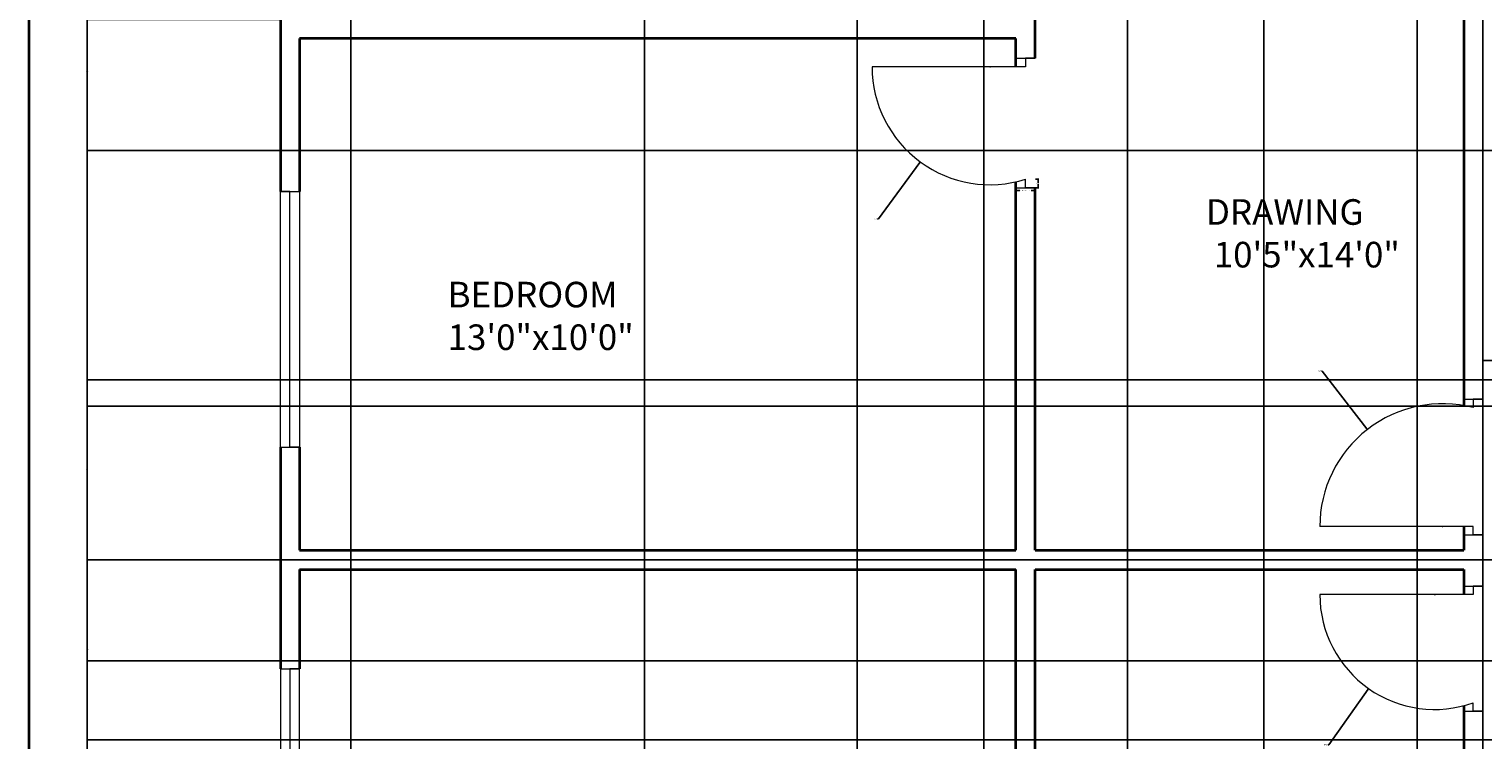
# Model space of a CAD drawing. Units: inches. Extents: x 1831 to 2867, y 1605 to 2524.
# Tile 3 of 7: x 1831 to 2172, y 2049 to 2216. Entities that reach past the tile are written whole.
import ezdxf

# ---------------------------------------------------------------- set-up
doc = ezdxf.new("R2010")
doc.units = ezdxf.units.IN
for name, color, linetype, lineweight in [('A-ANNO-DIMS', 2, 'Continuous', 18), ('A-ANNO-TTLB', 7, 'Continuous', 35), ('A-AREA-IDEN', 7, 'Continuous', 18), ('A-DOOR', 11, 'Continuous', 18), ('A-GLAZ', 121, 'Continuous', 18), ('A-WALL', 7, 'Continuous', 35)]:
    doc.layers.add(name, color=color, linetype=linetype, lineweight=lineweight)
doc.styles.get("Standard").update_dxf_attribs({"font": 'arial.ttf'})
doc.dimstyles.get("Standard").update_dxf_attribs({"dimtxt": 0.18, "dimasz": 0.18, "dimexe": 0.18, "dimexo": 0.0625, "dimgap": 0.09, "dimtad": 0, "dimtih": 1, "dimtoh": 1, "dimdec": 4, "dimzin": 0, "dimdsep": 46, "dimtxsty": 'Standard', "dimcen": 0.09, "dimadec": 0, "dimazin": 0, "dimtfac": 1, "dimtdec": 4, "dimtofl": 0, "dimtmove": 0, "dimatfit": 3, "dimfxl": 1, "dimtolj": 1, "dimtzin": 0, "dimarcsym": 0})

# ---------------------------------------------------------------- blocks, each defined once
blk = doc.blocks.new('WIN-60IN')
for p, q in [((4.5, 60), (0, 60)), ((0, 60), (2.25, 60)), ((0, 0), (0, 60)), ((2.25, 60), (2.25, 0)), ((4.5, 60), (4.5, 0)), ((4.5, 0), (0, 0)), ((2.25, 0), (4.5, 0))]:
    blk.add_line(p, q)
blk = doc.blocks.new('DOOR-LEAF-36IN-ALT')
for p, q in [((36, 2), (0, 2)), ((33.75, 0), (38.25, 0)), ((36, 0), (36, 2)), ((38.25, 0), (36, 0))]:
    blk.add_line(p, q)
blk = doc.blocks.new('DOOR-STRIKE-JAMB')
for p, q in [((0, 0), (4.5, 0)), ((2.25, 0), (2.25, 2)), ((4.5, 0), (2.25, 0))]:
    blk.add_line(p, q)
blk = doc.blocks.new('*D10')
at = {"layer": 'A-ANNO-DIMS', "color": 0, "lineweight": -2, "transparency": 16777216}
for p, q in [((2062.55, 2178.63), (2062.55, 2177.84)), ((2067.05, 2178.63), (2067.05, 2177.84)), ((2062.73, 2178.02), (2063.48, 2178.02)), ((2066.87, 2178.02), (2066.12, 2178.02))]:
    blk.add_line(p, q, dxfattribs=at)
at = {"layer": 'A-ANNO-DIMS', "color": 0, "transparency": 16777216}
for points in [[(2062.73, 2178.05), (2062.73, 2177.99), (2062.55, 2178.02)], [(2066.87, 2178.05), (2066.87, 2177.99), (2067.05, 2178.02)]]:
    blk.add_solid(points, dxfattribs=at)
at = {"layer": 'Defpoints', "color": 0, "transparency": 16777216}
for p in [(2062.55, 2178.7), (2067.05, 2178.7), (2067.05, 2178.02)]:
    blk.add_point(p, dxfattribs=at)
at = {"layer": 'A-ANNO-DIMS', "color": 0, "transparency": 16777216, "insert": (2064.8, 2178.02), "char_height": 0.18, "attachment_point": 5}
blk.add_mtext('\\A1;STRIKE JAMB 5 TYP.', dxfattribs=at)
blk = doc.blocks.new('*D11')
at = {"layer": 'A-ANNO-DIMS', "color": 0, "lineweight": -2, "transparency": 16777216}
for p, q in [((2067.11, 2180.7), (2067.91, 2180.7)), ((2067.11, 2178.7), (2067.91, 2178.7)), ((2067.73, 2180.52), (2067.73, 2179.88)), ((2067.73, 2178.88), (2067.73, 2179.52))]:
    blk.add_line(p, q, dxfattribs=at)
at = {"layer": 'A-ANNO-DIMS', "color": 0, "transparency": 16777216}
for points in [[(2067.7, 2180.52), (2067.76, 2180.52), (2067.73, 2180.7)], [(2067.7, 2178.88), (2067.76, 2178.88), (2067.73, 2178.7)]]:
    blk.add_solid(points, dxfattribs=at)
at = {"layer": 'Defpoints', "color": 0, "transparency": 16777216}
for p in [(2067.05, 2180.7), (2067.05, 2178.7), (2067.73, 2180.7)]:
    blk.add_point(p, dxfattribs=at)
at = {"layer": 'A-ANNO-DIMS', "color": 0, "transparency": 16777216, "insert": (2067.73, 2179.7), "char_height": 0.18, "attachment_point": 5}
blk.add_mtext('\\A1;2 TYP.', dxfattribs=at)
blk = doc.blocks.new('*D33')
at = {"layer": 'A-ANNO-DIMS', "color": 0, "lineweight": -2, "transparency": 16777216}
for p, q in [((1889.99, 2218.17), (1844.57, 2218.17)), ((1844.75, 2217.99), (1844.75, 2093.86)), ((1844.75, 1969.35), (1844.75, 2093.49)), ((1889.99, 1969.17), (1844.57, 1969.17))]:
    blk.add_line(p, q, dxfattribs=at)
at = {"layer": 'A-ANNO-DIMS', "color": 0, "transparency": 16777216}
for points in [[(1844.72, 2217.99), (1844.78, 2217.99), (1844.75, 2218.17)], [(1844.72, 1969.35), (1844.78, 1969.35), (1844.75, 1969.17)]]:
    blk.add_solid(points, dxfattribs=at)
at = {"layer": 'Defpoints', "color": 0, "transparency": 16777216}
for p in [(1890.05, 2218.17), (1844.75, 1969.17), (1890.05, 1969.17)]:
    blk.add_point(p, dxfattribs=at)
at = {"layer": 'A-ANNO-DIMS', "color": 0, "transparency": 16777216, "insert": (1844.75, 2093.67), "char_height": 0.18, "attachment_point": 5}
blk.add_mtext('\\A1;249', dxfattribs=at)
blk = doc.blocks.new('*D37')
at = {"layer": 'A-ANNO-DIMS', "color": 0, "lineweight": -2, "transparency": 16777216}
for p, q in [((1906.55, 2387.11), (1906.55, 1715.69)), ((1975.47, 2387.11), (1975.47, 1715.69)), ((1906.73, 1715.87), (1940.62, 1715.87)), ((1975.29, 1715.87), (1941.4, 1715.87))]:
    blk.add_line(p, q, dxfattribs=at)
at = {"layer": 'A-ANNO-DIMS', "color": 0, "transparency": 16777216}
for points in [[(1906.73, 1715.9), (1906.73, 1715.84), (1906.55, 1715.87)], [(1975.29, 1715.9), (1975.29, 1715.84), (1975.47, 1715.87)]]:
    blk.add_solid(points, dxfattribs=at)
at = {"layer": 'Defpoints', "color": 0, "transparency": 16777216}
for p in [(1906.55, 2387.17), (1975.47, 2387.17), (1975.47, 1715.87)]:
    blk.add_point(p, dxfattribs=at)
at = {"layer": 'A-ANNO-DIMS', "color": 0, "transparency": 16777216, "insert": (1941.01, 1715.87), "char_height": 0.18, "attachment_point": 5}
blk.add_mtext('\\A1;68.92', dxfattribs=at)
blk = doc.blocks.new('*D38')
at = {"layer": 'A-ANNO-DIMS', "color": 0, "lineweight": -2, "transparency": 16777216}
for p, q in [((1975.47, 2391.61), (1975.47, 1715.69)), ((2025.28, 2391.61), (2025.28, 1715.69)), ((1975.65, 1715.87), (1999.99, 1715.87)), ((2025.1, 1715.87), (2000.75, 1715.87))]:
    blk.add_line(p, q, dxfattribs=at)
at = {"layer": 'A-ANNO-DIMS', "color": 0, "transparency": 16777216}
for points in [[(1975.65, 1715.9), (1975.65, 1715.84), (1975.47, 1715.87)], [(2025.1, 1715.9), (2025.1, 1715.84), (2025.28, 1715.87)]]:
    blk.add_solid(points, dxfattribs=at)
at = {"layer": 'Defpoints', "color": 0, "transparency": 16777216}
for p in [(1975.47, 2391.67), (2025.28, 2391.67), (2025.28, 1715.87)]:
    blk.add_point(p, dxfattribs=at)
at = {"layer": 'A-ANNO-DIMS', "color": 0, "transparency": 16777216, "insert": (2000.37, 1715.87), "char_height": 0.18, "attachment_point": 5}
blk.add_mtext('\\A1;49.81', dxfattribs=at)
blk = doc.blocks.new('*D39')
at = {"layer": 'A-ANNO-DIMS', "color": 0, "lineweight": -2, "transparency": 16777216}
for p, q in [((2055.05, 2387.11), (2055.05, 1715.69)), ((2088.73, 2387.11), (2088.73, 1715.69)), ((2055.23, 1715.87), (2071.5, 1715.87)), ((2088.55, 1715.87), (2072.28, 1715.87))]:
    blk.add_line(p, q, dxfattribs=at)
at = {"layer": 'A-ANNO-DIMS', "color": 0, "transparency": 16777216}
for points in [[(2055.23, 1715.9), (2055.23, 1715.84), (2055.05, 1715.87)], [(2088.55, 1715.9), (2088.55, 1715.84), (2088.73, 1715.87)]]:
    blk.add_solid(points, dxfattribs=at)
at = {"layer": 'Defpoints', "color": 0, "transparency": 16777216}
for p in [(2055.05, 2387.17), (2088.73, 2387.17), (2088.73, 1715.87)]:
    blk.add_point(p, dxfattribs=at)
at = {"layer": 'A-ANNO-DIMS', "color": 0, "transparency": 16777216, "insert": (2071.89, 1715.87), "char_height": 0.18, "attachment_point": 5}
blk.add_mtext('\\A1;33.68', dxfattribs=at)
blk = doc.blocks.new('*D40')
at = {"layer": 'A-ANNO-DIMS', "color": 0, "lineweight": -2, "transparency": 16777216}
for p, q in [((2088.73, 2387.11), (2088.73, 1715.69)), ((2120.64, 2387.11), (2120.64, 1715.69)), ((2088.91, 1715.87), (2104.31, 1715.87)), ((2120.46, 1715.87), (2105.06, 1715.87))]:
    blk.add_line(p, q, dxfattribs=at)
at = {"layer": 'A-ANNO-DIMS', "color": 0, "transparency": 16777216}
for points in [[(2088.91, 1715.9), (2088.91, 1715.84), (2088.73, 1715.87)], [(2120.46, 1715.9), (2120.46, 1715.84), (2120.64, 1715.87)]]:
    blk.add_solid(points, dxfattribs=at)
at = {"layer": 'Defpoints', "color": 0, "transparency": 16777216}
for p in [(2088.73, 2387.17), (2120.64, 2387.17), (2120.64, 1715.87)]:
    blk.add_point(p, dxfattribs=at)
at = {"layer": 'A-ANNO-DIMS', "color": 0, "transparency": 16777216, "insert": (2104.69, 1715.87), "char_height": 0.18, "attachment_point": 5}
blk.add_mtext('\\A1;31.91', dxfattribs=at)
blk = doc.blocks.new('*D41')
at = {"layer": 'A-ANNO-DIMS', "color": 0, "lineweight": -2, "transparency": 16777216}
for p, q in [((2156.64, 2387.11), (2156.64, 1715.69)), ((2210.17, 2387.11), (2210.17, 1715.69)), ((2156.82, 1715.87), (2183.01, 1715.87)), ((2209.99, 1715.87), (2183.8, 1715.87))]:
    blk.add_line(p, q, dxfattribs=at)
at = {"layer": 'A-ANNO-DIMS', "color": 0, "transparency": 16777216}
for points in [[(2156.82, 1715.9), (2156.82, 1715.84), (2156.64, 1715.87)], [(2209.99, 1715.9), (2209.99, 1715.84), (2210.17, 1715.87)]]:
    blk.add_solid(points, dxfattribs=at)
at = {"layer": 'Defpoints', "color": 0, "transparency": 16777216}
for p in [(2156.64, 2387.17), (2210.17, 2387.17), (2210.17, 1715.87)]:
    blk.add_point(p, dxfattribs=at)
at = {"layer": 'A-ANNO-DIMS', "color": 0, "transparency": 16777216, "insert": (2183.4, 1715.87), "char_height": 0.18, "attachment_point": 5}
blk.add_mtext('\\A1;53.52', dxfattribs=at)
blk = doc.blocks.new('*D51')
at = {"layer": 'A-ANNO-DIMS', "color": 0, "lineweight": -2, "transparency": 16777216}
for p, q in [((2786.99, 2224.6), (1844.57, 2224.6)), ((1844.75, 2224.42), (1844.75, 2206.21)), ((1844.75, 2187.63), (1844.75, 2205.85)), ((2786.99, 2187.45), (1844.57, 2187.45))]:
    blk.add_line(p, q, dxfattribs=at)
at = {"layer": 'A-ANNO-DIMS', "color": 0, "transparency": 16777216}
for points in [[(1844.72, 2224.42), (1844.78, 2224.42), (1844.75, 2224.6)], [(1844.72, 2187.63), (1844.78, 2187.63), (1844.75, 2187.45)]]:
    blk.add_solid(points, dxfattribs=at)
at = {"layer": 'Defpoints', "color": 0, "transparency": 16777216}
for p in [(2787.05, 2224.6), (1844.75, 2187.45), (2787.05, 2187.45)]:
    blk.add_point(p, dxfattribs=at)
at = {"layer": 'A-ANNO-DIMS', "color": 0, "transparency": 16777216, "insert": (1844.75, 2206.03), "char_height": 0.18, "attachment_point": 5}
blk.add_mtext('\\A1;37.15', dxfattribs=at)
blk = doc.blocks.new('*D52')
at = {"layer": 'A-ANNO-DIMS', "color": 0, "lineweight": -2, "transparency": 16777216}
for p, q in [((2786.99, 2127.45), (1844.57, 2127.45)), ((1844.75, 2127.27), (1844.75, 2097.76)), ((1844.75, 2067.88), (1844.75, 2097.39)), ((2786.99, 2067.7), (1844.57, 2067.7))]:
    blk.add_line(p, q, dxfattribs=at)
at = {"layer": 'A-ANNO-DIMS', "color": 0, "transparency": 16777216}
for points in [[(1844.72, 2127.27), (1844.78, 2127.27), (1844.75, 2127.45)], [(1844.72, 2067.88), (1844.78, 2067.88), (1844.75, 2067.7)]]:
    blk.add_solid(points, dxfattribs=at)
at = {"layer": 'Defpoints', "color": 0, "transparency": 16777216}
for p in [(2787.05, 2127.45), (1844.75, 2067.7), (2787.05, 2067.7)]:
    blk.add_point(p, dxfattribs=at)
at = {"layer": 'A-ANNO-DIMS', "color": 0, "transparency": 16777216, "insert": (1844.75, 2097.57), "char_height": 0.18, "attachment_point": 5}
blk.add_mtext('\\A1;59.76', dxfattribs=at)
blk = doc.blocks.new('*D60')
at = {"layer": 'A-ANNO-DIMS', "color": 0, "lineweight": -2, "transparency": 16777216}
for p, q in [((2225.43, 2091.42), (1844.57, 2091.42)), ((1844.75, 2091.24), (1844.75, 2070.48)), ((1844.75, 2049.35), (1844.75, 2070.12)), ((2225.43, 2049.17), (1844.57, 2049.17))]:
    blk.add_line(p, q, dxfattribs=at)
at = {"layer": 'A-ANNO-DIMS', "color": 0, "transparency": 16777216}
for points in [[(1844.72, 2091.24), (1844.78, 2091.24), (1844.75, 2091.42)], [(1844.72, 2049.35), (1844.78, 2049.35), (1844.75, 2049.17)]]:
    blk.add_solid(points, dxfattribs=at)
at = {"layer": 'Defpoints', "color": 0, "transparency": 16777216}
for p in [(1844.75, 2091.42), (2225.49, 2091.42), (2225.49, 2049.17)]:
    blk.add_point(p, dxfattribs=at)
at = {"layer": 'A-ANNO-DIMS', "color": 0, "transparency": 16777216, "insert": (1844.75, 2070.3), "char_height": 0.18, "attachment_point": 5}
blk.add_mtext('\\A1;42.25', dxfattribs=at)
blk = doc.blocks.new('*D61')
at = {"layer": 'A-ANNO-DIMS', "color": 0, "lineweight": -2, "transparency": 16777216}
for p, q in [((2225.43, 2133.67), (1844.57, 2133.67)), ((1844.75, 2133.49), (1844.75, 2112.73)), ((1844.75, 2091.6), (1844.75, 2112.37)), ((2225.43, 2091.42), (1844.57, 2091.42))]:
    blk.add_line(p, q, dxfattribs=at)
at = {"layer": 'A-ANNO-DIMS', "color": 0, "transparency": 16777216}
for points in [[(1844.72, 2133.49), (1844.78, 2133.49), (1844.75, 2133.67)], [(1844.72, 2091.6), (1844.78, 2091.6), (1844.75, 2091.42)]]:
    blk.add_solid(points, dxfattribs=at)
at = {"layer": 'Defpoints', "color": 0, "transparency": 16777216}
for p in [(1844.75, 2133.67), (2225.49, 2133.67), (2225.49, 2091.42)]:
    blk.add_point(p, dxfattribs=at)
at = {"layer": 'A-ANNO-DIMS', "color": 0, "transparency": 16777216, "insert": (1844.75, 2112.55), "char_height": 0.18, "attachment_point": 5}
blk.add_mtext('\\A1;42.25', dxfattribs=at)
blk = doc.blocks.new('*D63')
at = {"layer": 'A-ANNO-DIMS', "color": 0, "lineweight": -2, "transparency": 16777216}
for p, q in [((2172.05, 1795.74), (2172.05, 2467.15)), ((2172.23, 2466.97), (2183.83, 2466.97)), ((2195.87, 2466.97), (2184.27, 2466.97)), ((2196.05, 1795.74), (2196.05, 2467.15))]:
    blk.add_line(p, q, dxfattribs=at)
at = {"layer": 'A-ANNO-DIMS', "color": 0, "transparency": 16777216}
for points in [[(2172.23, 2467), (2172.23, 2466.94), (2172.05, 2466.97)], [(2195.87, 2467), (2195.87, 2466.94), (2196.05, 2466.97)]]:
    blk.add_solid(points, dxfattribs=at)
at = {"layer": 'Defpoints', "color": 0, "transparency": 16777216}
for p in [(2196.05, 2466.97), (2172.05, 1795.67), (2196.05, 1795.67)]:
    blk.add_point(p, dxfattribs=at)
at = {"layer": 'A-ANNO-DIMS', "color": 0, "transparency": 16777216, "insert": (2184.05, 2466.97), "char_height": 0.18, "attachment_point": 5}
blk.add_mtext('\\A1;24', dxfattribs=at)
blk = doc.blocks.new('*D64')
at = {"layer": 'A-ANNO-DIMS', "color": 0, "lineweight": -2, "transparency": 16777216}
for p, q in [((2172.11, 2138.17), (2838.45, 2138.17)), ((2838.27, 2137.99), (2838.27, 2136.11)), ((2838.27, 2133.85), (2838.27, 2135.74)), ((2172.11, 2133.67), (2838.45, 2133.67))]:
    blk.add_line(p, q, dxfattribs=at)
at = {"layer": 'A-ANNO-DIMS', "color": 0, "transparency": 16777216}
for points in [[(2838.24, 2137.99), (2838.3, 2137.99), (2838.27, 2138.17)], [(2838.24, 2133.85), (2838.3, 2133.85), (2838.27, 2133.67)]]:
    blk.add_solid(points, dxfattribs=at)
at = {"layer": 'Defpoints', "color": 0, "transparency": 16777216}
for p in [(2172.05, 2138.17), (2172.05, 2133.67), (2838.27, 2133.67)]:
    blk.add_point(p, dxfattribs=at)
at = {"layer": 'A-ANNO-DIMS', "color": 0, "transparency": 16777216, "insert": (2838.27, 2135.92), "char_height": 0.18, "attachment_point": 5}
blk.add_mtext('\\A1;4.5', dxfattribs=at)
blk = doc.blocks.new('*D70')
at = {"layer": 'A-ANNO-DIMS', "color": 0, "lineweight": -2, "transparency": 16777216}
for p, q in [((2134.21, 2135.67), (2134.39, 2135.67)), ((2134.39, 2135.67), (2144.86, 2122.15)), ((2162.5, 2099.25), (2162.68, 2099.25)), ((2162.59, 2099.16), (2162.59, 2099.34))]:
    blk.add_line(p, q, dxfattribs=at)
at = {"layer": 'A-ANNO-DIMS', "color": 0, "transparency": 16777216}
blk.add_solid([(2144.88, 2122.17), (2144.83, 2122.13), (2144.97, 2122.01)], dxfattribs=at)
at = {"layer": 'Defpoints', "color": 0, "transparency": 16777216}
for p in [(2144.97, 2122.01), (2162.59, 2099.25)]:
    blk.add_point(p, dxfattribs=at)
at = {"layer": 'A-ANNO-DIMS', "color": 0, "transparency": 16777216, "insert": (2133.73, 2135.67), "char_height": 0.18, "attachment_point": 5}
blk.add_mtext('\\A1;R28.79', dxfattribs=at)
blk = doc.blocks.new('*D76')
at = {"layer": 'A-ANNO-DIMS', "color": 0, "lineweight": -2, "transparency": 16777216}
for p, q in [((2056.39, 2207.09), (2056.57, 2207.09)), ((2056.48, 2207), (2056.48, 2207.18)), ((2030.29, 2171.38), (2040.01, 2184.63)), ((2030.11, 2171.38), (2030.29, 2171.38))]:
    blk.add_line(p, q, dxfattribs=at)
at = {"layer": 'A-ANNO-DIMS', "color": 0, "transparency": 16777216}
blk.add_solid([(2039.98, 2184.65), (2040.03, 2184.61), (2040.11, 2184.77)], dxfattribs=at)
at = {"layer": 'Defpoints', "color": 0, "transparency": 16777216}
for p in [(2056.48, 2207.09), (2040.11, 2184.77)]:
    blk.add_point(p, dxfattribs=at)
at = {"layer": 'A-ANNO-DIMS', "color": 0, "transparency": 16777216, "insert": (2029.63, 2171.38), "char_height": 0.18, "attachment_point": 5}
blk.add_mtext('\\A1;R27.68', dxfattribs=at)
blk = doc.blocks.new('*D79')
at = {"layer": 'A-ANNO-DIMS', "color": 0, "lineweight": -2, "transparency": 16777216}
for p, q in [((2160.66, 2083.26), (2160.84, 2083.26)), ((2160.75, 2083.17), (2160.75, 2083.35)), ((2135.91, 2048.03), (2145.12, 2061.09)), ((2135.73, 2048.03), (2135.91, 2048.03))]:
    blk.add_line(p, q, dxfattribs=at)
at = {"layer": 'A-ANNO-DIMS', "color": 0, "transparency": 16777216}
blk.add_solid([(2145.09, 2061.11), (2145.14, 2061.08), (2145.22, 2061.24)], dxfattribs=at)
at = {"layer": 'Defpoints', "color": 0, "transparency": 16777216}
for p in [(2160.75, 2083.26), (2145.22, 2061.24)]:
    blk.add_point(p, dxfattribs=at)
at = {"layer": 'A-ANNO-DIMS', "color": 0, "transparency": 16777216, "insert": (2135.18, 2048.03), "char_height": 0.18, "attachment_point": 5}
blk.add_mtext('\\A1;R26.945', dxfattribs=at)

msp = doc.modelspace()

# ---------------------------------------------------------------- linework, layer by layer
at = {"layer": 'A-ANNO-TTLB'}
msp.add_lwpolyline([(1831.1248, 2523.9204), (2867.0416, 2523.9204), (2867.0416, 1605.0781), (1831.1248, 1605.0781)], close=True, dxfattribs=at)
at = {"layer": 'A-DOOR'}
for centre, radius, start, end in [((2056.4795, 2207.0936), 27.6785, 180, 287.49653), ((2162.593, 2099.2455), 28.792, 75.501832, 180), ((2160.7458, 2083.2638), 26.9447, 180, 289.63746)]:
    msp.add_arc(centre, radius, start, end, dxfattribs=at)
at = {"layer": 'A-WALL'}
for p, q in [((2167.551, 2256.6738), (2167.551, 2127.6074)), ((1890.051, 2218.1738), (1890.051, 2177.8352)), ((2067.051, 2213.6738), (2067.051, 2218.1738)), ((1906.551, 2213.6738), (1894.551, 2213.6738)), ((1894.551, 2213.6738), (1894.551, 2177.8352)), ((2007.051, 2213.6738), (1906.551, 2213.6738)), ((2062.551, 2213.6738), (2007.051, 2213.6738)), ((2062.551, 2207.0936), (2062.551, 2213.6738)), ((2067.051, 2209.0936), (2067.051, 2213.6738)), ((2062.551, 2093.6738), (2062.551, 2180.0892)), ((2067.051, 2093.6738), (2067.051, 2178.6956)), ((1890.051, 2117.8352), (1890.051, 2098.1738)), ((1894.551, 2117.8352), (1894.551, 2093.6738)), ((1890.051, 2098.1738), (1890.051, 2089.1738)), ((2167.551, 2099.2455), (2167.551, 2093.6738)), ((1894.551, 2093.6738), (1906.551, 2093.6738)), ((1906.551, 2093.6738), (2062.551, 2093.6738)), ((2067.051, 2093.6738), (2167.551, 2093.6738)), ((1890.051, 2089.1738), (1890.051, 2065.8506)), ((1894.551, 2089.1738), (2062.551, 2089.1738)), ((1894.551, 2089.1738), (1894.551, 2065.8506)), ((1906.551, 2089.1738), (2062.551, 2089.1738)), ((2062.551, 2002.7385), (2062.551, 2089.1738)), ((2067.051, 2003.8704), (2067.051, 2089.1738)), ((2067.051, 2089.1738), (2167.551, 2089.1738)), ((2067.051, 2089.1738), (2167.551, 2089.1738)), ((2167.551, 2089.1738), (2167.551, 2083.2638)), ((2167.551, 2057.1926), (2167.551, 1926.1738))]:
    msp.add_line(p, q, dxfattribs=at)

# ---------------------------------------------------------------- block references
at = {"layer": 'A-DOOR', "extrusion": (0, 0, -1), "zscale": -1, "rotation": 180}
for name, p in [('DOOR-LEAF-36IN-ALT', (-2028.801, 2209.0936)), ('DOOR-STRIKE-JAMB', (-2167.551, 2129.1206)), ('DOOR-LEAF-36IN-ALT', (-2133.801, 2085.2638))]:
    msp.add_blockref(name, p, dxfattribs=at)
at = {"layer": 'A-DOOR'}
for name, p in [('DOOR-STRIKE-JAMB', (2062.551, 2178.6956)), ('DOOR-LEAF-36IN-ALT', (2133.801, 2097.2455)), ('DOOR-STRIKE-JAMB', (2167.551, 2055.8862))]:
    msp.add_blockref(name, p, dxfattribs=at)
at = {"layer": 'A-GLAZ', "rotation": 180}
msp.add_blockref('WIN-60IN', (1894.551, 2177.8352), dxfattribs=at)
at = {"layer": 'A-GLAZ', "extrusion": (0, 0, -1), "zscale": -1}
msp.add_blockref('WIN-60IN', (-1894.551, 2005.8506), dxfattribs=at)

# ---------------------------------------------------------------- texts
at = {"layer": 'A-AREA-IDEN', "char_height": 6, "attachment_point": 1}
for s, width, insert in [('DRAWING\\P 10\'5"x14\'0"', 177.829253, (2107.1008, 2176.0134)), ('BEDROOM\\P13\'0"x10\'0"', 142.639935, (1929.2777, 2156.6402))]:
    msp.add_mtext_dynamic_manual_height_columns(s, width=width, gutter_width=12.5, heights=[0], dxfattribs=dict(at, insert=insert))

# ---------------------------------------------------------------- dimensions: what is measured, and where the dimension line sits
at = {"layer": 'A-ANNO-DIMS'}
for base, p1, p2, override, picture, middle in [((2196.051, 2466.9738), (2172.051, 1795.6738), (2196.051, 1795.6738), {"dimdec": 0, "dimlfac": 1, "dimrnd": 0, "dimzin": 0, "dimdsep": 46, "dimlunit": 2}, '*D63', (2184.051, 2466.9738)), ((2025.2753, 1715.8738), (1975.4676, 2391.6738), (2025.2753, 2391.6738), {"dimdec": 2, "dimlfac": 1, "dimrnd": 0, "dimzin": 0, "dimdsep": 46, "dimlunit": 2}, '*D38', (2000.3714, 1715.8738)), ((1975.4676, 1715.8738), (1906.551, 2387.1738), (1975.4676, 2387.1738), {"dimdec": 2, "dimlfac": 1, "dimrnd": 0, "dimzin": 0, "dimdsep": 46, "dimlunit": 2}, '*D37', (1941.0093, 1715.8738)), ((2088.7306, 1715.8738), (2055.051, 2387.1738), (2088.7306, 2387.1738), {"dimdec": 2, "dimlfac": 1, "dimrnd": 0, "dimzin": 0, "dimdsep": 46, "dimlunit": 2}, '*D39', (2071.8908, 1715.8738)), ((2120.6429, 1715.8738), (2088.7306, 2387.1738), (2120.6429, 2387.1738), {"dimdec": 2, "dimlfac": 1, "dimrnd": 0, "dimzin": 0, "dimdsep": 46, "dimlunit": 2}, '*D40', (2104.6867, 1715.8738)), ((2210.1653, 1715.8738), (2156.6429, 2387.1738), (2210.1653, 2387.1738), {"dimdec": 2, "dimlfac": 1, "dimrnd": 0, "dimzin": 0, "dimdsep": 46, "dimlunit": 2}, '*D41', (2183.4041, 1715.8738))]:
    dim = msp.add_linear_dim(base=base, p1=p1, p2=p2, dimstyle='Standard', override=override, dxfattribs=at)
    dim.commit()
    dim.dimension.update_dxf_attribs({"geometry": picture, "text_midpoint": middle})
for base, p1, p2, override, picture, middle in [((1844.751, 2187.452), (2787.051, 2224.6027), (2787.051, 2187.452), {"dimdec": 2, "dimlfac": 1, "dimrnd": 0, "dimzin": 0, "dimdsep": 46, "dimlunit": 2}, '*D51', (1844.751, 2206.0273)), ((1844.751, 1969.1738), (1890.051, 2218.1738), (1890.051, 1969.1738), {"dimdec": 0, "dimlfac": 1, "dimrnd": 0, "dimzin": 0, "dimdsep": 46, "dimlunit": 2}, '*D33', (1844.751, 2093.6738)), ((2838.2663, 2133.6738), (2172.051, 2138.1738), (2172.051, 2133.6738), {"dimdec": 1, "dimlfac": 1, "dimrnd": 0, "dimzin": 0, "dimdsep": 46, "dimlunit": 2}, '*D64', (2838.2663, 2135.9238)), ((1844.751, 2133.6738), (2225.4925, 2091.4238), (2225.4925, 2133.6738), {"dimdec": 2, "dimlfac": 1, "dimrnd": 0, "dimzin": 0, "dimdsep": 46, "dimlunit": 2}, '*D61', (1844.751, 2112.5488)), ((1844.751, 2067.6955), (2787.051, 2127.452), (2787.051, 2067.6955), {"dimdec": 2, "dimlfac": 1, "dimrnd": 0, "dimzin": 0, "dimdsep": 46, "dimlunit": 2}, '*D52', (1844.751, 2097.5738)), ((1844.751, 2091.4238), (2225.4925, 2049.1738), (2225.4925, 2091.4238), {"dimdec": 2, "dimlfac": 1, "dimrnd": 0, "dimzin": 0, "dimdsep": 46, "dimlunit": 2}, '*D60', (1844.751, 2070.2988))]:
    dim = msp.add_linear_dim(base=base, p1=p1, p2=p2, angle=90, dimstyle='Standard', override=override, dxfattribs=at)
    dim.commit()
    dim.dimension.update_dxf_attribs({"geometry": picture, "text_midpoint": middle})
for center, mpoint, override, picture, middle in [((2056.4795, 2207.0936), (2040.1121, 2184.7731), {"dimdec": 2, "dimlfac": 1, "dimrnd": 0, "dimzin": 0, "dimdsep": 46, "dimlunit": 2}, '*D76', (2029.6316, 2171.3808)), ((2162.593, 2099.2455), (2144.966, 2122.011), {"dimdec": 2, "dimlfac": 1, "dimrnd": 0, "dimzin": 0, "dimdsep": 46, "dimlunit": 2}, '*D70', (2133.7298, 2135.6703)), ((2160.7458, 2083.2638), (2145.221, 2061.241), {"dimdec": 3, "dimlfac": 1, "dimrnd": 0, "dimzin": 0, "dimdsep": 46, "dimlunit": 2}, '*D79', (2135.1757, 2048.0274))]:
    dim = msp.add_radius_dim(center=center, mpoint=mpoint, dimstyle='Standard', override=override, dxfattribs=at)
    dim.commit()
    dim.dimension.update_dxf_attribs({"geometry": picture, "text_midpoint": middle, "dimtype": 164})
dim = msp.add_linear_dim(base=(2067.0510031976, 2178.0206467776), p1=(2062.5510031976, 2178.6956467776), p2=(2067.0510031976, 2178.6956467776), text='STRIKE JAMB <> TYP.', dimstyle='Standard', override={"dimdec": 0, "dimlfac": 1, "dimrnd": 0, "dimzin": 0, "dimdsep": 46, "dimlunit": 2}, dxfattribs=at)
dim.commit()
dim.dimension.update_dxf_attribs({"geometry": '*D10', "text_midpoint": (2064.8010031976, 2178.0206467776)})
dim = msp.add_linear_dim(base=(2067.726, 2180.6956), p1=(2067.051, 2178.6956), p2=(2067.051, 2180.6956), angle=90, text='<> TYP.', dimstyle='Standard', override={"dimdec": 0, "dimlfac": 1, "dimrnd": 0, "dimzin": 0, "dimdsep": 46, "dimlunit": 2}, dxfattribs=at)
dim.commit()
dim.dimension.update_dxf_attribs({"geometry": '*D11', "text_midpoint": (2067.726, 2179.6956)})

doc.saveas('drawing.dxf')
